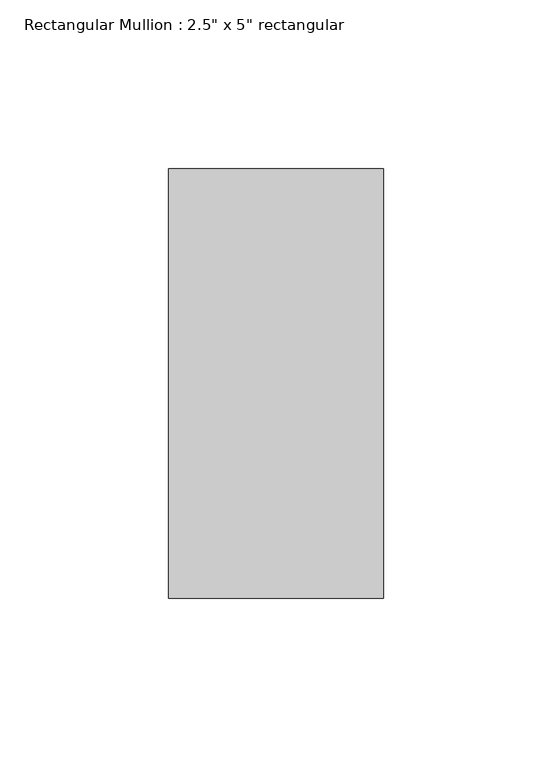
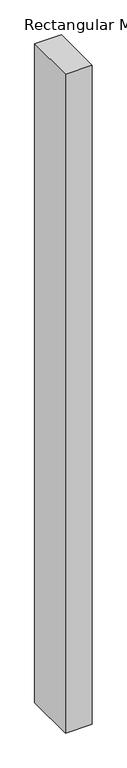
"""IFC4 building model written with IfcOpenShell, lengths in millimetres: member geometry."""

from ifc_helpers import new_model, si_unit, frame, origin, place, context, project, spatial, polyline, outline, extrude, source, transform, mapped, element, save


def member_4c0b5a72(model_context):
    return source(origin(), model_context, "Body", "SweptSolid", [
        extrude(outline(polyline([(31.75, 63.5), (31.75, -63.5), (-31.75, -63.5), (-31.75, 63.5), (31.75, 63.5)])), frame((0.0, 0.0, -1659.4287133), z_axis=(0.0, 0.0, 1.0), x_axis=(1.0, 0.0, 0.0)), (0.0, 0.0, 1.0), 1659.4287133),
    ])


if __name__ == "__main__":
    model = new_model("IFC4")
    model_context = context("Model", 3, world=origin())
    ifc_project = project(units=[si_unit("LENGTHUNIT", "METRE", prefix="MILLI")], contexts=[model_context])
    site = spatial("IfcSite", under=ifc_project)
    building = spatial("IfcBuilding", under=site)
    placement = place(None, origin())
    member_shape = member_4c0b5a72(model_context)
    element("IfcMember", 1, ObjectType="Rectangular Mullion : 2.5\" x 5\" rectangular", at=placement, inside=building, context=model_context, shape_type="MappedRepresentation", body=[
        mapped(member_shape, transform((0.0, 0.0, 0.0), x_axis=(1.0, 0.0, 0.0), y_axis=(0.0, 1.0, 0.0), z_axis=(0.0, 0.0, 1.0))),
    ])
    save(model, "model.ifc")

# Revit data of these elements
# Type "Rectangular Mullion : 2.5\" x 5\" rectangular"
#   built-in parameter 1007304 = 0.416667 (stored number, unit not read)
#   built-in parameter 1007301 = 0.104167 (stored number, unit not read)
#   built-in parameter 1007300 = 0.104167 (stored number, unit not read)
# Element 1 (IfcMember, "Rectangular Mullion : 2.5\" x 5\" rectangular")
#   Materials on its faces: "Aluminum"
# Materials
#   "Aluminum": class "Metal", colour RGB 247 247 247, transparency 0, Description = "Aluminum 6061", Cost = 0
